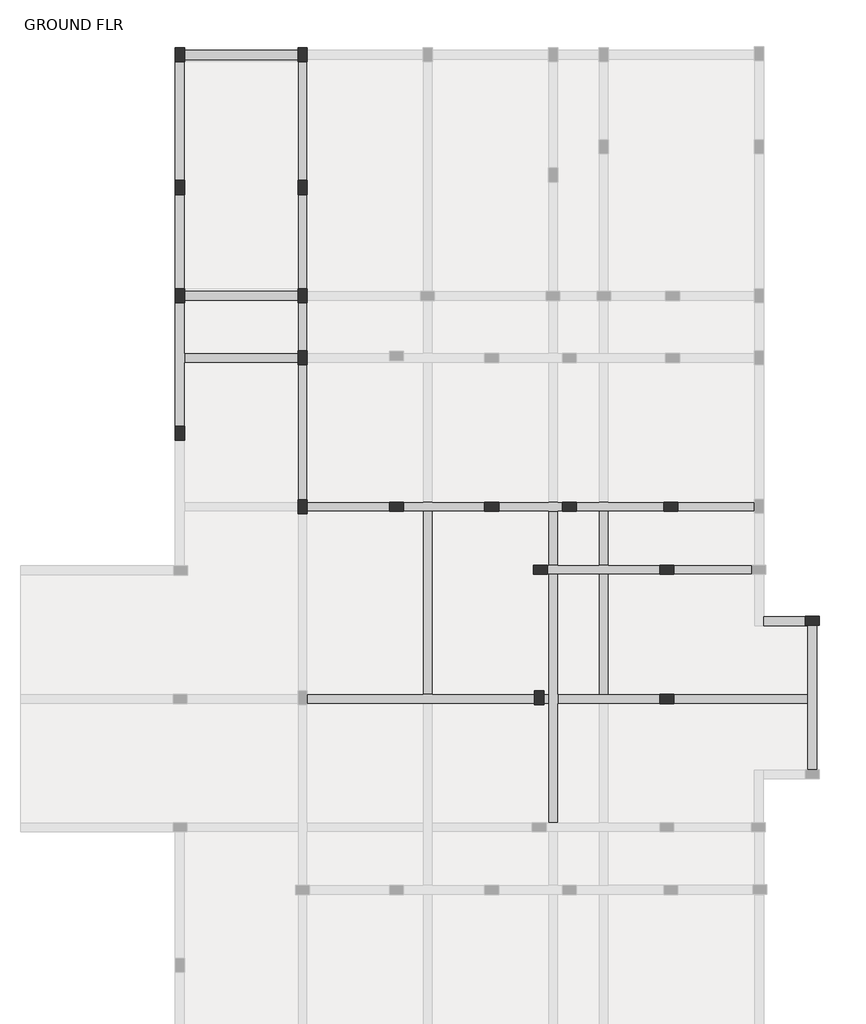
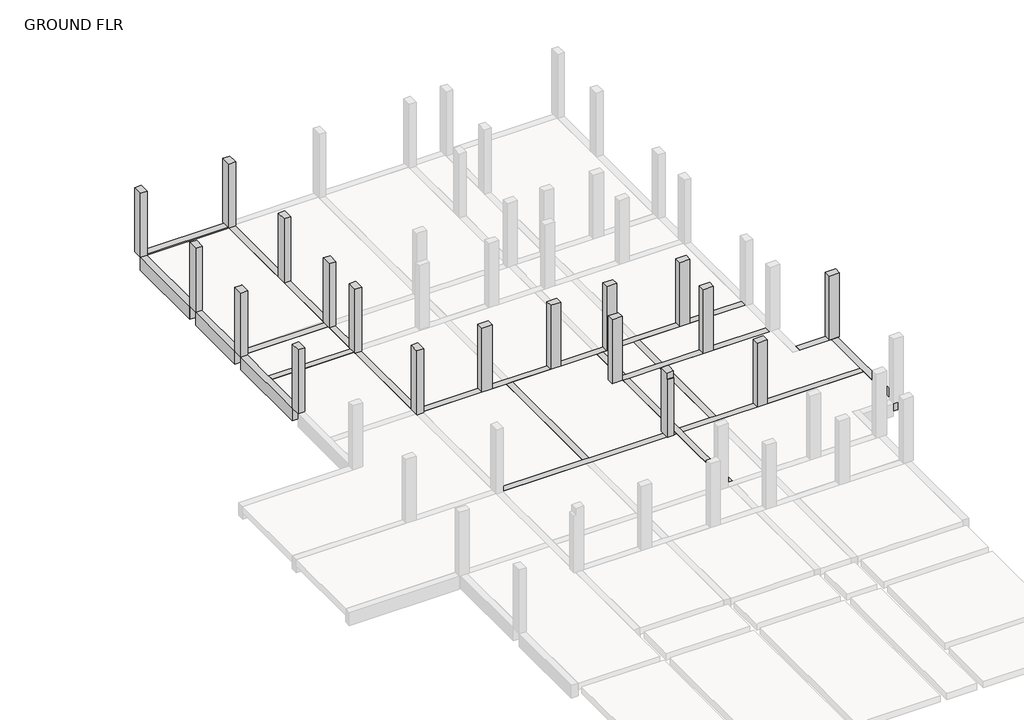
# One storey, part 4 of 5: 29 beams, 18 columns.
"""IFC4 building model written with IfcOpenShell, lengths in millimetres."""

from ifc_helpers import new_model, si_unit, frame, origin, origin_with_axes, place, context, project, spatial, polyline, outline, extrude, faceted_brep, element, save

model = new_model("IFC4")

# Units and contexts
model_context = context("Model", 3, world=origin())
ifc_project = project(units=[si_unit("LENGTHUNIT", "METRE", prefix="MILLI")], contexts=[model_context])

# Site, building, storey
site = spatial("IfcSite", under=ifc_project)
building = spatial("IfcBuilding", under=site)
storey = spatial("IfcBuildingStorey", under=building, Name="GROUND FLR", Elevation=0.0)

# Beams
placement = place(None, origin())
element("IfcBeam", 1, ObjectType="M_Concrete-Rectangular Beam : 300 x 600mm", at=placement, inside=storey, context=model_context, shape_type="SweptSolid", body=[
    extrude(outline(polyline([(-1971.7865686, 21837.8349362), (-1971.7865686, 21537.8349362), (-5591.7865686, 21537.8349362), (-5591.7865686, 21837.8349362), (-1971.7865686, 21837.8349362)])), frame((0.0, 0.0, -600.0), z_axis=(0.0, 0.0, 1.0), x_axis=(1.0, 0.0, 0.0)), (0.0, 0.0, 1.0), 600.0),
])
element("IfcBeam", 2, ObjectType="M_Concrete-Rectangular Beam : 300 x 600mm", at=placement, inside=storey, context=model_context, shape_type="Brep", body=[
    faceted_brep([(-5891.7865686, 21462.8349362, 0.0), (-5891.7865686, 17662.8349362, 0.0), (-5888.8105653, 17662.8349362, 0.0), (-5888.8105653, 17674.7148651, 0.0), (-5591.7865686, 17674.7148651, 0.0), (-5591.7865686, 21462.8349362, 0.0), (-5891.7865686, 21462.8349362, -600.0), (-5891.7865686, 17662.8349362, -600.0), (-5591.7865686, 21462.8349362, -600.0), (-5591.7865686, 17674.7148651, -600.0), (-5888.8105653, 17674.7148651, -600.0), (-5888.8105653, 17662.8349362, -600.0), (-5591.7865686, 17674.7148651, -300.0), (-5591.7865686, 21462.8349362, -300.0)], [[[0, 1, 2, 3, 4, 5]], [[1, 0, 6, 7]], [[7, 6, 8, 9, 10, 11]], [[5, 4, 12, 9, 8, 13]], [[8, 6, 0, 5, 13]], [[1, 7, 11, 2]], [[10, 3, 2, 11]], [[3, 10, 9, 12, 4]]]),
])
element("IfcBeam", 3, ObjectType="M_Concrete-Rectangular Beam : 300 x 600mm", at=placement, inside=storey, context=model_context, shape_type="SweptSolid", body=[
    extrude(outline(polyline([(0.0, -5888.8105653), (-600.0, -5888.8105653), (-600.0, -5588.8105653), (-300.0, -5588.8105653), (-300.0, -5591.7865686), (0.0, -5591.7865686), (0.0, -5888.8105653)])), frame((0.0, 14212.5179708, 0.0), z_axis=(0.0, 1.0, 0.0), x_axis=(0.0, 0.0, 1.0)), (0.0, 0.0, 1.0), 3012.1968944),
])
element("IfcBeam", 4, ObjectType="M_Concrete-Rectangular Beam : 300 x 600mm", at=placement, inside=storey, context=model_context, shape_type="Brep", body=[
    faceted_brep([(-5888.8105653, 13762.5179708, 0.0), (-5888.8105653, 9817.5252033, 0.0), (-5588.8105653, 9817.5252033, 0.0), (-5588.8105653, 11857.4075451, 0.0), (-5588.8105653, 12157.4075451, 0.0), (-5588.8105653, 13762.5179708, 0.0), (-5888.8105653, 13762.5179708, -600.0), (-5888.8105653, 9817.5252033, -600.0), (-5588.8105653, 13762.5179708, -600.0), (-5588.8105653, 12157.4075451, -600.0), (-5588.8105653, 11857.4075451, -600.0), (-5588.8105653, 9817.5252033, -600.0), (-5588.8105653, 13762.5179708, -300.0), (-5588.8105653, 9817.5252033, -300.0)], [[[0, 1, 2, 3, 4, 5]], [[1, 0, 6, 7]], [[7, 6, 8, 9, 10, 11]], [[11, 10, 9, 8, 12, 5, 4, 3, 2, 13]], [[8, 6, 0, 5, 12]], [[2, 1, 7, 11, 13]]]),
])
element("IfcBeam", 5, ObjectType="M_Concrete-Rectangular Beam : 300 x 600mm", at=placement, inside=storey, context=model_context, shape_type="Brep", body=[
    faceted_brep([(14319.1163908, 3443.0536525, 0.0), (14619.1163908, 3443.0536525, 0.0), (14619.1163908, 3443.0536525, -600.0), (14319.1163908, 3443.0536525, -600.0), (14319.1163908, 3435.7536525, 0.0), (14319.1163908, 1251.1713929, 0.0), (14319.1163908, 951.1713929, 0.0), (14319.1163908, -1148.8286071, 0.0), (14619.1163908, -1148.8286071, 0.0), (14619.1163908, -1148.8286071, -600.0), (14319.1163908, -1148.8286071, -600.0), (14319.1163908, 951.1713929, -600.0), (14319.1163908, 1251.1713929, -600.0), (14319.1163908, 3435.7536525, -600.0), (14319.1163908, -1148.8286071, -300.0)], [[[0, 1, 2, 3]], [[1, 0, 4, 5, 6, 7, 8]], [[2, 1, 8, 9]], [[3, 2, 9, 10, 11, 12, 13]], [[0, 3, 13, 12, 11, 10, 14, 7, 6, 5, 4]], [[7, 14, 10, 9, 8]]]),
])
element("IfcBeam", 6, ObjectType="M_Concrete-Rectangular Beam : 300 x 600mm", at=placement, inside=storey, context=model_context, shape_type="Brep", body=[
    faceted_brep([(12916.8679014, 3735.7536525, 0.0), (12916.8679014, 3435.7536525, 0.0), (14319.1163908, 3435.7536525, 0.0), (14319.1163908, 3443.0536525, 0.0), (14619.1163908, 3443.0536525, 0.0), (14619.1163908, 3455.7536525, 0.0), (14244.1163908, 3455.7536525, 0.0), (14244.1163908, 3735.7536525, 0.0), (12916.8679014, 3735.7536525, -600.0), (14244.1163908, 3735.7536525, -600.0), (12916.8679014, 3435.7536525, -600.0), (14244.1163908, 3455.7536525, -600.0), (14619.1163908, 3455.7536525, -600.0), (14619.1163908, 3443.0536525, -600.0), (14319.1163908, 3443.0536525, -600.0), (14319.1163908, 3435.7536525, -600.0), (12916.8679014, 3435.7536525, -300.0), (14319.1163908, 3435.7536525, -300.0)], [[[0, 1, 2, 3, 4, 5, 6, 7]], [[8, 0, 7, 9]], [[10, 8, 9, 11, 12, 13, 14, 15]], [[2, 1, 16, 10, 15, 17]], [[1, 0, 8, 10, 16]], [[12, 5, 4, 13]], [[7, 6, 11, 9]], [[11, 6, 5, 12]], [[3, 14, 13, 4]], [[14, 3, 2, 17, 15]]]),
])
element("IfcBeam", 7, ObjectType="M_Concrete-Rectangular Beam : 300 x 600mm", at=placement, inside=storey, context=model_context, shape_type="Brep", body=[
    faceted_brep([(-1671.7865686, 21462.8349362, 0.0), (-1971.7865686, 21462.8349362, 0.0), (-1971.7865686, 17674.7148651, 0.0), (-1671.7865686, 17674.7148651, 0.0), (-1971.7865686, 21462.8349362, -300.0), (-1971.7865686, 21462.8349362, -600.0), (-1971.7865686, 17674.7148651, -600.0), (-1971.7865686, 17674.7148651, -300.0), (-1671.7865686, 21462.8349362, -600.0), (-1671.7865686, 17674.7148651, -600.0), (-1671.7865686, 17674.7148651, -300.0), (-1671.7865686, 21462.8349362, -300.0)], [[[0, 1, 2, 3]], [[2, 1, 4, 5, 6, 7]], [[5, 8, 9, 6]], [[0, 3, 10, 9, 8, 11]], [[1, 0, 11, 8, 5, 4]], [[3, 2, 7, 6, 9, 10]]]),
])
element("IfcBeam", 8, ObjectType="M_Concrete-Rectangular Beam : 300 x 600mm", at=placement, inside=storey, context=model_context, shape_type="Brep", body=[
    faceted_brep([(-1671.7865686, 17224.7148651, 0.0), (-1971.7865686, 17224.7148651, 0.0), (-1971.7865686, 14212.5179708, 0.0), (-1671.7865686, 14212.5179708, 0.0), (-1971.7865686, 17224.7148651, -300.0), (-1971.7865686, 17224.7148651, -600.0), (-1971.7865686, 14212.5179708, -600.0), (-1971.7865686, 14212.5179708, -300.0), (-1671.7865686, 17224.7148651, -600.0), (-1671.7865686, 14212.5179708, -600.0), (-1671.7865686, 14212.5179708, -300.0), (-1671.7865686, 17224.7148651, -300.0)], [[[0, 1, 2, 3]], [[2, 1, 4, 5, 6, 7]], [[5, 8, 9, 6]], [[0, 3, 10, 9, 8, 11]], [[1, 0, 11, 8, 5, 4]], [[3, 2, 7, 6, 9, 10]]]),
])
element("IfcBeam", 9, ObjectType="M_Concrete-Rectangular Beam : 300 x 600mm", at=placement, inside=storey, context=model_context, shape_type="Brep", body=[
    faceted_brep([(-1671.7865686, 13762.5179708, 0.0), (-1971.7865686, 13762.5179708, 0.0), (-1971.7865686, 12232.4075451, 0.0), (-1671.7865686, 12232.4075451, 0.0), (-1971.7865686, 13762.5179708, -300.0), (-1971.7865686, 13762.5179708, -600.0), (-1971.7865686, 12232.4075451, -600.0), (-1971.7865686, 12232.4075451, -300.0), (-1671.7865686, 13762.5179708, -600.0), (-1671.7865686, 12232.4075451, -600.0), (-1671.7865686, 12232.4075451, -300.0), (-1671.7865686, 13762.5179708, -300.0)], [[[0, 1, 2, 3]], [[2, 1, 4, 5, 6, 7]], [[5, 8, 9, 6]], [[0, 3, 10, 9, 8, 11]], [[1, 0, 11, 8, 5, 4]], [[3, 2, 7, 6, 9, 10]]]),
])
element("IfcBeam", 10, ObjectType="M_Concrete-Rectangular Beam : 300 x 600mm", at=placement, inside=storey, context=model_context, shape_type="Brep", body=[
    faceted_brep([(-1671.7865686, 11782.4075451, 0.0), (-1971.7865686, 11782.4075451, 0.0), (-1971.7865686, 7474.7076276, 0.0), (-1671.7865686, 7474.7076276, 0.0), (-1971.7865686, 11782.4075451, -300.0), (-1971.7865686, 11782.4075451, -600.0), (-1971.7865686, 7474.7076276, -600.0), (-1971.7865686, 7474.7076276, -300.0), (-1671.7865686, 11782.4075451, -600.0), (-1671.7865686, 7474.7076276, -600.0), (-1671.7865686, 7474.7076276, -300.0), (-1671.7865686, 11782.4075451, -300.0)], [[[0, 1, 2, 3]], [[2, 1, 4, 5, 6, 7]], [[5, 8, 9, 6]], [[0, 3, 10, 9, 8, 11]], [[1, 0, 11, 8, 5, 4]], [[3, 2, 7, 6, 9, 10]]]),
])
element("IfcBeam", 11, ObjectType="M_Concrete-Rectangular Beam : 300 x 600mm", at=placement, inside=storey, context=model_context, shape_type="Brep", body=[
    faceted_brep([(-5588.8105653, 14137.5179708, 0.0), (-5588.8105653, 13837.5179708, 0.0), (-1971.7865686, 13837.5179708, 0.0), (-1971.7865686, 14137.5179708, 0.0), (-5588.8105653, 13837.5179708, -300.0), (-5588.8105653, 13837.5179708, -600.0), (-1971.7865686, 13837.5179708, -600.0), (-1971.7865686, 13837.5179708, -300.0), (-5588.8105653, 14137.5179708, -600.0), (-1971.7865686, 14137.5179708, -600.0)], [[[0, 1, 2, 3]], [[2, 1, 4, 5, 6, 7]], [[5, 8, 9, 6]], [[8, 0, 3, 9]], [[1, 0, 8, 5, 4]], [[9, 3, 2, 7, 6]]]),
])
element("IfcBeam", 12, ObjectType="M_Concrete-Rectangular Beam : 300 x 600mm", at=placement, inside=storey, context=model_context, shape_type="Brep", body=[
    faceted_brep([(-1971.7865686, 11857.4075451, 0.0), (-1971.7865686, 12157.4075451, 0.0), (-5588.8105653, 12157.4075451, 0.0), (-5588.8105653, 11857.4075451, 0.0), (-5588.8105653, 11857.4075451, -300.0), (-5588.8105653, 11857.4075451, -600.0), (-1971.7865686, 11857.4075451, -600.0), (-1971.7865686, 11857.4075451, -300.0), (-1971.7865686, 12157.4075451, -600.0), (-5588.8105653, 12157.4075451, -600.0), (-1971.7865686, 12157.4075451, -300.0), (-5588.8105653, 12157.4075451, -300.0)], [[[0, 1, 2, 3]], [[0, 3, 4, 5, 6, 7]], [[8, 6, 5, 9]], [[2, 1, 10, 8, 9, 11]], [[1, 0, 7, 6, 8, 10]], [[3, 2, 11, 9, 5, 4]]]),
])
element("IfcBeam", 13, ObjectType="M_Concrete-Rectangular Beam : 300 x 600mm", at=placement, inside=storey, context=model_context, shape_type="Brep", body=[
    faceted_brep([(-1671.7865686, 7399.7076276, 0.0), (-1671.7865686, 7099.7076276, 0.0), (949.7296816, 7099.7076276, 0.0), (949.7296816, 7399.7076276, 0.0), (-1671.7865686, 7099.7076276, -300.0), (-1671.7865686, 7099.7076276, -600.0), (949.7296816, 7099.7076276, -600.0), (949.7296816, 7099.7076276, -300.0), (-1671.7865686, 7399.7076276, -600.0), (949.7296816, 7399.7076276, -600.0), (949.7296816, 7399.7076276, -300.0), (-1671.7865686, 7399.7076276, -300.0)], [[[0, 1, 2, 3]], [[2, 1, 4, 5, 6, 7]], [[5, 8, 9, 6]], [[0, 3, 10, 9, 8, 11]], [[1, 0, 11, 8, 5, 4]], [[3, 2, 7, 6, 9, 10]]]),
])
element("IfcBeam", 14, ObjectType="M_Concrete-Rectangular Beam : 300 x 600mm", at=placement, inside=storey, context=model_context, shape_type="Brep", body=[
    faceted_brep([(1399.7296816, 7399.7076276, 0.0), (1399.7296816, 7099.7076276, 0.0), (2024.7296816, 7099.7076276, 0.0), (2324.7296816, 7099.7076276, 0.0), (3997.5248054, 7099.7076276, 0.0), (3997.5248054, 7399.7076276, 0.0), (2324.7296816, 7399.7076276, 0.0), (2024.7296816, 7399.7076276, 0.0), (1399.7296816, 7099.7076276, -600.0), (2024.7296816, 7099.7076276, -600.0), (2324.7296816, 7099.7076276, -600.0), (3997.5248054, 7099.7076276, -600.0), (3997.5248054, 7099.7076276, -300.0), (1399.7296816, 7099.7076276, -300.0), (1399.7296816, 7399.7076276, -600.0), (2024.7296816, 7399.7076276, -600.0), (2324.7296816, 7399.7076276, -600.0), (3997.5248054, 7399.7076276, -600.0), (1399.7296816, 7399.7076276, -300.0), (3997.5248054, 7399.7076276, -300.0)], [[[0, 1, 2, 3, 4, 5, 6, 7]], [[8, 9, 10, 11, 12, 4, 3, 2, 1, 13]], [[8, 14, 15, 16, 17, 11, 10, 9]], [[17, 16, 15, 14, 18, 0, 7, 6, 5, 19]], [[1, 0, 18, 14, 8, 13]], [[5, 4, 12, 11, 17, 19]]]),
])
element("IfcBeam", 15, ObjectType="M_Concrete-Rectangular Beam : 300 x 600mm", at=placement, inside=storey, context=model_context, shape_type="Brep", body=[
    faceted_brep([(4447.5248054, 7399.7076276, 0.0), (4447.5248054, 7099.7076276, 0.0), (6032.5248054, 7099.7076276, 0.0), (6332.5248054, 7099.7076276, 0.0), (6481.8679014, 7099.7076276, 0.0), (6481.8679014, 7399.7076276, 0.0), (6332.5248054, 7399.7076276, 0.0), (6032.5248054, 7399.7076276, 0.0), (4447.5248054, 7099.7076276, -600.0), (6032.5248054, 7099.7076276, -600.0), (6332.5248054, 7099.7076276, -600.0), (6481.8679014, 7099.7076276, -600.0), (6481.8679014, 7099.7076276, -300.0), (4447.5248054, 7099.7076276, -300.0), (4447.5248054, 7399.7076276, -600.0), (6032.5248054, 7399.7076276, -600.0), (6332.5248054, 7399.7076276, -600.0), (6481.8679014, 7399.7076276, -600.0), (4447.5248054, 7399.7076276, -300.0), (6481.8679014, 7399.7076276, -300.0)], [[[0, 1, 2, 3, 4, 5, 6, 7]], [[8, 9, 10, 11, 12, 4, 3, 2, 1, 13]], [[8, 14, 15, 16, 17, 11, 10, 9]], [[17, 16, 15, 14, 18, 0, 7, 6, 5, 19]], [[1, 0, 18, 14, 8, 13]], [[5, 4, 12, 11, 17, 19]]]),
])
element("IfcBeam", 16, ObjectType="M_Concrete-Rectangular Beam : 300 x 600mm", at=placement, inside=storey, context=model_context, shape_type="Brep", body=[
    faceted_brep([(6931.8679014, 7399.7076276, 0.0), (6931.8679014, 7099.7076276, 0.0), (7656.8679014, 7099.7076276, 0.0), (7956.8679014, 7099.7076276, 0.0), (9721.8679014, 7099.7076276, 0.0), (9721.8679014, 7399.7076276, 0.0), (7956.8679014, 7399.7076276, 0.0), (7656.8679014, 7399.7076276, 0.0), (6931.8679014, 7099.7076276, -600.0), (7656.8679014, 7099.7076276, -600.0), (7956.8679014, 7099.7076276, -600.0), (9721.8679014, 7099.7076276, -600.0), (9721.8679014, 7099.7076276, -300.0), (6931.8679014, 7099.7076276, -300.0), (6931.8679014, 7399.7076276, -600.0), (7656.8679014, 7399.7076276, -600.0), (7956.8679014, 7399.7076276, -600.0), (9721.8679014, 7399.7076276, -600.0), (6931.8679014, 7399.7076276, -300.0), (9721.8679014, 7399.7076276, -300.0)], [[[0, 1, 2, 3, 4, 5, 6, 7]], [[8, 9, 10, 11, 12, 4, 3, 2, 1, 13]], [[8, 14, 15, 16, 17, 11, 10, 9]], [[17, 16, 15, 14, 18, 0, 7, 6, 5, 19]], [[1, 0, 18, 14, 8, 13]], [[5, 4, 12, 11, 17, 19]]]),
])
element("IfcBeam", 17, ObjectType="M_Concrete-Rectangular Beam : 300 x 600mm", at=placement, inside=storey, context=model_context, shape_type="Brep", body=[
    faceted_brep([(6007.5248054, 5387.6057249, 0.0), (6007.5248054, 5087.6057249, 0.0), (6032.5248054, 5087.6057249, 0.0), (6332.5248054, 5087.6057249, 0.0), (7656.8679014, 5087.6057249, 0.0), (7956.8679014, 5087.6057249, 0.0), (9601.8679014, 5087.6057249, 0.0), (9601.8679014, 5387.6057249, 0.0), (7956.8679014, 5387.6057249, 0.0), (7656.8679014, 5387.6057249, 0.0), (6332.5248054, 5387.6057249, 0.0), (6032.5248054, 5387.6057249, 0.0), (6007.5248054, 5087.6057249, -600.0), (6032.5248054, 5087.6057249, -600.0), (6332.5248054, 5087.6057249, -600.0), (7656.8679014, 5087.6057249, -600.0), (7956.8679014, 5087.6057249, -600.0), (9601.8679014, 5087.6057249, -600.0), (9601.8679014, 5087.6057249, -300.0), (6007.5248054, 5087.6057249, -300.0), (6007.5248054, 5387.6057249, -600.0), (6032.5248054, 5387.6057249, -600.0), (6332.5248054, 5387.6057249, -600.0), (7656.8679014, 5387.6057249, -600.0), (7956.8679014, 5387.6057249, -600.0), (9601.8679014, 5387.6057249, -600.0), (6007.5248054, 5387.6057249, -300.0), (9601.8679014, 5387.6057249, -300.0)], [[[0, 1, 2, 3, 4, 5, 6, 7, 8, 9, 10, 11]], [[12, 13, 14, 15, 16, 17, 18, 6, 5, 4, 3, 2, 1, 19]], [[12, 20, 21, 22, 23, 24, 25, 17, 16, 15, 14, 13]], [[25, 24, 23, 22, 21, 20, 26, 0, 11, 10, 9, 8, 7, 27]], [[1, 0, 26, 20, 12, 19]], [[7, 6, 18, 17, 25, 27]]]),
])
element("IfcBeam", 18, ObjectType="M_Concrete-Rectangular Beam : 300 x 600mm", at=placement, inside=storey, context=model_context, shape_type="Brep", body=[
    faceted_brep([(10051.8679014, 5387.6057249, 0.0), (10051.8679014, 5087.6057249, 0.0), (12541.8679014, 5087.6057249, 0.0), (12541.8679014, 5387.6057249, 0.0), (10051.8679014, 5087.6057249, -300.0), (10051.8679014, 5087.6057249, -600.0), (12541.8679014, 5087.6057249, -600.0), (12541.8679014, 5087.6057249, -300.0), (10051.8679014, 5387.6057249, -600.0), (12541.8679014, 5387.6057249, -600.0), (12541.8679014, 5387.6057249, -300.0), (10051.8679014, 5387.6057249, -300.0)], [[[0, 1, 2, 3]], [[2, 1, 4, 5, 6, 7]], [[5, 8, 9, 6]], [[0, 3, 10, 9, 8, 11]], [[1, 0, 11, 8, 5, 4]], [[3, 2, 7, 6, 9, 10]]]),
])
element("IfcBeam", 19, ObjectType="M_Concrete-Rectangular Beam : 300 x 600mm", at=placement, inside=storey, context=model_context, shape_type="Brep", body=[
    faceted_brep([(10051.8679014, 1251.1713929, 0.0), (10051.8679014, 951.1713929, 0.0), (14319.1163908, 951.1713929, 0.0), (14319.1163908, 1251.1713929, 0.0), (10051.8679014, 951.1713929, -300.0), (10051.8679014, 951.1713929, -600.0), (14319.1163908, 951.1713929, -600.0), (14319.1163908, 951.1713929, -300.0), (10051.8679014, 1251.1713929, -600.0), (14319.1163908, 1251.1713929, -600.0), (14319.1163908, 1251.1713929, -300.0), (10051.8679014, 1251.1713929, -300.0)], [[[0, 1, 2, 3]], [[2, 1, 4, 5, 6, 7]], [[5, 8, 9, 6]], [[0, 3, 10, 9, 8, 11]], [[1, 0, 11, 8, 5, 4]], [[3, 2, 7, 6, 9, 10]]]),
])
element("IfcBeam", 20, ObjectType="M_Concrete-Rectangular Beam : 300 x 600mm", at=placement, inside=storey, context=model_context, shape_type="Brep", body=[
    faceted_brep([(6032.5248054, 951.1713929, 0.0), (6032.5248054, 1251.1713929, 0.0), (5892.5248054, 1251.1713929, 0.0), (5892.5248054, 951.1713929, 0.0), (5892.5248054, 951.1713929, -300.0), (5892.5248054, 951.1713929, -600.0), (6032.5248054, 951.1713929, -600.0), (6032.5248054, 951.1713929, -300.0), (6032.5248054, 1251.1713929, -600.0), (5892.5248054, 1251.1713929, -600.0), (6032.5248054, 1251.1713929, -300.0), (5892.5248054, 1251.1713929, -300.0)], [[[0, 1, 2, 3]], [[0, 3, 4, 5, 6, 7]], [[8, 6, 5, 9]], [[2, 1, 10, 8, 9, 11]], [[1, 0, 7, 6, 8, 10]], [[3, 2, 11, 9, 5, 4]]]),
    faceted_brep([(-1671.7865686, 951.1713929, 0.0), (-1671.7865686, 1251.1713929, 0.0), (-1671.7865686, 1251.1713929, -300.0), (-1671.7865686, 1251.1713929, -600.0), (-1671.7865686, 951.1713929, -600.0), (-1671.7865686, 951.1713929, -300.0), (5592.5248054, 1251.1713929, 0.0), (5592.5248054, 951.1713929, 0.0), (5592.5248054, 951.1713929, -300.0), (5592.5248054, 951.1713929, -600.0), (5592.5248054, 1251.1713929, -600.0), (5592.5248054, 1251.1713929, -300.0), (2024.7296816, 951.1713929, 0.0), (2324.7296816, 951.1713929, 0.0), (2324.7296816, 1251.1713929, 0.0), (2024.7296816, 1251.1713929, 0.0), (2024.7296816, 951.1713929, -600.0), (2324.7296816, 951.1713929, -600.0), (2024.7296816, 1251.1713929, -600.0), (2324.7296816, 1251.1713929, -600.0)], [[[0, 1, 2, 3, 4, 5]], [[6, 7, 8, 9, 10, 11]], [[1, 0, 12, 13, 7, 6, 14, 15]], [[4, 16, 17, 9, 8, 7, 13, 12, 0, 5]], [[4, 3, 18, 19, 10, 9, 17, 16]], [[10, 19, 18, 3, 2, 1, 15, 14, 6, 11]]]),
])
element("IfcBeam", 21, ObjectType="M_Concrete-Rectangular Beam : 300 x 600mm", at=placement, inside=storey, context=model_context, shape_type="Brep", body=[
    faceted_brep([(2324.7296816, 7099.7076276, 0.0), (2024.7296816, 7099.7076276, 0.0), (2024.7296816, 1251.1713929, 0.0), (2324.7296816, 1251.1713929, 0.0), (2024.7296816, 7099.7076276, -300.0), (2024.7296816, 7099.7076276, -600.0), (2024.7296816, 1251.1713929, -600.0), (2024.7296816, 1251.1713929, -300.0), (2324.7296816, 7099.7076276, -600.0), (2324.7296816, 5387.6057249, -600.0), (2324.7296816, 5087.6057249, -600.0), (2324.7296816, 1251.1713929, -600.0), (2324.7296816, 1251.1713929, -300.0), (2324.7296816, 7099.7076276, -300.0)], [[[0, 1, 2, 3]], [[2, 1, 4, 5, 6, 7]], [[5, 8, 9, 10, 11, 6]], [[0, 3, 12, 11, 10, 9, 8, 13]], [[1, 0, 13, 8, 5, 4]], [[3, 2, 7, 6, 11, 12]]]),
])
element("IfcBeam", 22, ObjectType="M_Concrete-Rectangular Beam : 300 x 600mm", at=placement, inside=storey, context=model_context, shape_type="Brep", body=[
    faceted_brep([(6332.5248054, 7099.7076276, 0.0), (6032.5248054, 7099.7076276, 0.0), (6032.5248054, 5387.6057249, 0.0), (6332.5248054, 5387.6057249, 0.0), (6032.5248054, 7099.7076276, -300.0), (6032.5248054, 7099.7076276, -600.0), (6032.5248054, 5387.6057249, -600.0), (6032.5248054, 5387.6057249, -300.0), (6332.5248054, 7099.7076276, -600.0), (6332.5248054, 5387.6057249, -600.0), (6332.5248054, 5387.6057249, -300.0), (6332.5248054, 7099.7076276, -300.0)], [[[0, 1, 2, 3]], [[2, 1, 4, 5, 6, 7]], [[5, 8, 9, 6]], [[0, 3, 10, 9, 8, 11]], [[1, 0, 11, 8, 5, 4]], [[3, 2, 7, 6, 9, 10]]]),
])
element("IfcBeam", 23, ObjectType="M_Concrete-Rectangular Beam : 300 x 600mm", at=placement, inside=storey, context=model_context, shape_type="Brep", body=[
    faceted_brep([(7956.8679014, 7099.7076276, 0.0), (7656.8679014, 7099.7076276, 0.0), (7656.8679014, 5387.6057249, 0.0), (7956.8679014, 5387.6057249, 0.0), (7656.8679014, 7099.7076276, -300.0), (7656.8679014, 7099.7076276, -600.0), (7656.8679014, 5387.6057249, -600.0), (7656.8679014, 5387.6057249, -300.0), (7956.8679014, 7099.7076276, -600.0), (7956.8679014, 5387.6057249, -600.0), (7956.8679014, 5387.6057249, -300.0), (7956.8679014, 7099.7076276, -300.0)], [[[0, 1, 2, 3]], [[2, 1, 4, 5, 6, 7]], [[5, 8, 9, 6]], [[0, 3, 10, 9, 8, 11]], [[1, 0, 11, 8, 5, 4]], [[3, 2, 7, 6, 9, 10]]]),
])
element("IfcBeam", 24, ObjectType="M_Concrete-Rectangular Beam : 300 x 600mm", at=placement, inside=storey, context=model_context, shape_type="Brep", body=[
    faceted_brep([(6332.5248054, 5087.6057249, 0.0), (6032.5248054, 5087.6057249, 0.0), (6032.5248054, 1251.1713929, 0.0), (6032.5248054, 951.1713929, 0.0), (6032.5248054, -2839.4535766, 0.0), (6332.5248054, -2839.4535766, 0.0), (6332.5248054, 951.1713929, 0.0), (6332.5248054, 1251.1713929, 0.0), (6032.5248054, 5087.6057249, -600.0), (6032.5248054, 1251.1713929, -600.0), (6032.5248054, 951.1713929, -600.0), (6032.5248054, -2839.4535766, -600.0), (6032.5248054, -2839.4535766, -300.0), (6032.5248054, 5087.6057249, -300.0), (6332.5248054, 5087.6057249, -600.0), (6332.5248054, 1251.1713929, -600.0), (6332.5248054, 951.1713929, -600.0), (6332.5248054, -2839.4535766, -600.0), (6332.5248054, 5087.6057249, -300.0), (6332.5248054, -2839.4535766, -300.0)], [[[0, 1, 2, 3, 4, 5, 6, 7]], [[8, 9, 10, 11, 12, 4, 3, 2, 1, 13]], [[8, 14, 15, 16, 17, 11, 10, 9]], [[17, 16, 15, 14, 18, 0, 7, 6, 5, 19]], [[1, 0, 18, 14, 8, 13]], [[5, 4, 12, 11, 17, 19]]]),
])
element("IfcBeam", 25, ObjectType="M_Concrete-Rectangular Beam : 300 x 600mm", at=placement, inside=storey, context=model_context, shape_type="Brep", body=[
    faceted_brep([(7956.8679014, 5087.6057249, 0.0), (7656.8679014, 5087.6057249, 0.0), (7656.8679014, 1251.1713929, 0.0), (7956.8679014, 1251.1713929, 0.0), (7656.8679014, 5087.6057249, -300.0), (7656.8679014, 5087.6057249, -600.0), (7656.8679014, 1251.1713929, -600.0), (7656.8679014, 1251.1713929, -300.0), (7956.8679014, 5087.6057249, -600.0), (7956.8679014, 1251.1713929, -600.0), (7956.8679014, 1251.1713929, -300.0), (7956.8679014, 5087.6057249, -300.0)], [[[0, 1, 2, 3]], [[2, 1, 4, 5, 6, 7]], [[5, 8, 9, 6]], [[0, 3, 10, 9, 8, 11]], [[1, 0, 11, 8, 5, 4]], [[3, 2, 7, 6, 9, 10]]]),
])
element("IfcBeam", 26, ObjectType="M_Concrete-Rectangular Beam : 300 x 600mm", at=placement, inside=storey, context=model_context, shape_type="Brep", body=[
    faceted_brep([(9601.8679014, 951.1713929, 0.0), (9601.8679014, 1251.1713929, 0.0), (7956.8679014, 1251.1713929, 0.0), (7656.8679014, 1251.1713929, 0.0), (6332.5248054, 1251.1713929, 0.0), (6332.5248054, 951.1713929, 0.0), (7656.8679014, 951.1713929, 0.0), (7956.8679014, 951.1713929, 0.0), (6332.5248054, 951.1713929, -600.0), (7656.8679014, 951.1713929, -600.0), (7956.8679014, 951.1713929, -600.0), (9601.8679014, 951.1713929, -600.0), (9601.8679014, 951.1713929, -300.0), (6332.5248054, 951.1713929, -300.0), (9601.8679014, 1251.1713929, -600.0), (6332.5248054, 1251.1713929, -600.0), (7656.8679014, 1251.1713929, -600.0), (7956.8679014, 1251.1713929, -600.0), (6332.5248054, 1251.1713929, -300.0), (9601.8679014, 1251.1713929, -300.0)], [[[0, 1, 2, 3, 4, 5, 6, 7]], [[8, 9, 10, 11, 12, 0, 7, 6, 5, 13]], [[14, 11, 10, 9, 8, 15, 16, 17]], [[14, 17, 16, 15, 18, 4, 3, 2, 1, 19]], [[1, 0, 12, 11, 14, 19]], [[5, 4, 18, 15, 8, 13]]]),
])
element("IfcBeam", 27, ObjectType="M_Concrete-Rectangular Beam : 300 x 600mm", at=placement, inside=storey, context=model_context, shape_type="Brep", body=[
    faceted_brep([(10171.8679014, 7399.7076276, 0.0), (10171.8679014, 7099.7076276, 0.0), (12616.8679014, 7099.7076276, 0.0), (12616.8679014, 7399.7076276, 0.0), (10171.8679014, 7099.7076276, -300.0), (10171.8679014, 7099.7076276, -600.0), (12616.8679014, 7099.7076276, -600.0), (12616.8679014, 7099.7076276, -300.0), (10171.8679014, 7399.7076276, -600.0), (12616.8679014, 7399.7076276, -600.0), (12616.8679014, 7399.7076276, -300.0), (10171.8679014, 7399.7076276, -300.0)], [[[0, 1, 2, 3]], [[2, 1, 4, 5, 6, 7]], [[5, 8, 9, 6]], [[0, 3, 10, 9, 8, 11]], [[8, 5, 4, 1, 0, 11]], [[3, 2, 7, 6, 9, 10]]]),
])
element("IfcBeam", 28, ObjectType="M_Concrete-Rectangular Beam : 300 x 600mm", at=placement, inside=storey, context=model_context, shape_type="SweptSolid", body=[
    extrude(outline(polyline([(2324.7296816, 5087.6057249), (2324.7296816, 5387.6057249), (2337.5248054, 5387.6057249), (2337.5248054, 5087.6057249), (2324.7296816, 5087.6057249)])), frame((0.0, 0.0, -600.0), z_axis=(0.0, 0.0, 1.0), x_axis=(1.0, 0.0, 0.0)), (0.0, 0.0, 1.0), 300.0),
])
element("IfcBeam", 29, ObjectType="M_Concrete-Rectangular Beam : 300 x 600mm", at=placement, inside=storey, context=model_context, shape_type="SweptSolid", body=[
    extrude(outline(polyline([(2337.5248054, 5087.6057249), (2337.5248054, 5387.6057249), (5557.5248054, 5387.6057249), (5557.5248054, 5087.6057249), (2337.5248054, 5087.6057249)])), frame((0.0, 0.0, -600.0), z_axis=(0.0, 0.0, 1.0), x_axis=(1.0, 0.0, 0.0)), (0.0, 0.0, 1.0), 300.0),
])

# Columns
element("IfcColumn", 30, ObjectType="M_Concrete-Rectangular-Column : 300 x 450mm", at=placement, inside=storey, context=model_context, shape_type="SweptSolid", body=[
    extrude(outline(polyline([(-5591.7865686, 21912.8349362), (-5591.7865686, 21462.8349362), (-5891.7865686, 21462.8349362), (-5891.7865686, 21912.8349362), (-5591.7865686, 21912.8349362)])), origin_with_axes(), (0.0, 0.0, 1.0), 3000.0),
])
element("IfcColumn", 31, ObjectType="M_Concrete-Rectangular-Column : 300 x 450mm", at=placement, inside=storey, context=model_context, shape_type="Brep", body=[
    faceted_brep([(-1671.7865686, 21912.8349362, 0.0), (-1671.7865686, 21462.8349362, 0.0), (-1971.7865686, 21462.8349362, 0.0), (-1971.7865686, 21912.8349362, 0.0), (-1671.7865686, 21912.8349362, 3000.0), (-1671.7865686, 21537.8349362, 3000.0), (-1671.7865686, 21462.8349362, 3000.0), (-1671.7865686, 21462.8349362, 2700.0), (-1971.7865686, 21462.8349362, 3000.0), (-1971.7865686, 21462.8349362, 2700.0), (-1971.7865686, 21912.8349362, 3000.0)], [[[0, 1, 2, 3]], [[1, 0, 4, 5, 6, 7]], [[2, 1, 7, 6, 8, 9]], [[3, 2, 9, 8, 10]], [[0, 3, 10, 4]], [[8, 6, 5, 4, 10]]]),
])
element("IfcColumn", 32, ObjectType="M_Concrete-Rectangular-Column : 300 x 450mm", at=placement, inside=storey, context=model_context, shape_type="Brep", body=[
    faceted_brep([(-1671.7865686, 17674.7148651, 0.0), (-1671.7865686, 17224.7148651, 0.0), (-1971.7865686, 17224.7148651, 0.0), (-1971.7865686, 17674.7148651, 0.0), (-1671.7865686, 17674.7148651, 2700.0), (-1671.7865686, 17674.7148651, 3000.0), (-1671.7865686, 17224.7148651, 3000.0), (-1671.7865686, 17224.7148651, 2700.0), (-1971.7865686, 17224.7148651, 3000.0), (-1971.7865686, 17224.7148651, 2700.0), (-1971.7865686, 17674.7148651, 3000.0), (-1971.7865686, 17674.7148651, 2700.0)], [[[0, 1, 2, 3]], [[1, 0, 4, 5, 6, 7]], [[2, 1, 7, 6, 8, 9]], [[3, 2, 9, 8, 10, 11]], [[0, 3, 11, 10, 5, 4]], [[6, 5, 10, 8]]]),
])
element("IfcColumn", 33, ObjectType="M_Concrete-Rectangular-Column : 300 x 450mm", at=placement, inside=storey, context=model_context, shape_type="SweptSolid", body=[
    extrude(outline(polyline([(0.0, -5888.8105653), (0.0, -5588.8105653), (2700.0, -5588.8105653), (2700.0, -5591.7865686), (3000.0, -5591.7865686), (3000.0, -5888.8105653), (0.0, -5888.8105653)])), frame((0.0, 17224.7148651, 0.0), z_axis=(0.0, 1.0, 0.0), x_axis=(0.0, 0.0, 1.0)), (0.0, 0.0, 1.0), 450.0),
])
element("IfcColumn", 34, ObjectType="M_Concrete-Rectangular-Column : 300 x 450mm", at=placement, inside=storey, context=model_context, shape_type="Brep", body=[
    faceted_brep([(-5588.8105653, 14212.5179708, 0.0), (-5588.8105653, 13762.5179708, 0.0), (-5888.8105653, 13762.5179708, 0.0), (-5888.8105653, 14212.5179708, 0.0), (-5588.8105653, 14212.5179708, 2700.0), (-5588.8105653, 14212.5179708, 3000.0), (-5588.8105653, 13837.5179708, 3000.0), (-5588.8105653, 13762.5179708, 3000.0), (-5588.8105653, 13762.5179708, 2700.0), (-5888.8105653, 13762.5179708, 3000.0), (-5888.8105653, 14212.5179708, 3000.0), (-5591.7865686, 14212.5179708, 3000.0)], [[[0, 1, 2, 3]], [[1, 0, 4, 5, 6, 7, 8]], [[2, 1, 8, 7, 9]], [[3, 2, 9, 10]], [[0, 3, 10, 11, 5, 4]], [[9, 7, 6, 5, 11, 10]]]),
])
element("IfcColumn", 35, ObjectType="M_Concrete-Rectangular-Column : 300 x 450mm", at=placement, inside=storey, context=model_context, shape_type="Brep", body=[
    faceted_brep([(-1671.7865686, 14212.5179708, 0.0), (-1671.7865686, 13762.5179708, 0.0), (-1971.7865686, 13762.5179708, 0.0), (-1971.7865686, 14212.5179708, 0.0), (-1671.7865686, 14212.5179708, 2700.0), (-1671.7865686, 14212.5179708, 3000.0), (-1671.7865686, 14137.5179708, 3000.0), (-1671.7865686, 13837.5179708, 3000.0), (-1671.7865686, 13762.5179708, 3000.0), (-1671.7865686, 13762.5179708, 2700.0), (-1971.7865686, 13762.5179708, 3000.0), (-1971.7865686, 13762.5179708, 2700.0), (-1971.7865686, 13837.5179708, 3000.0), (-1971.7865686, 14212.5179708, 3000.0), (-1971.7865686, 14212.5179708, 2700.0)], [[[0, 1, 2, 3]], [[1, 0, 4, 5, 6, 7, 8, 9]], [[2, 1, 9, 8, 10, 11]], [[3, 2, 11, 10, 12, 13, 14]], [[0, 3, 14, 13, 5, 4]], [[10, 8, 7, 6, 5, 13, 12]]]),
])
element("IfcColumn", 36, ObjectType="M_Concrete-Rectangular-Column : 300 x 450mm", at=placement, inside=storey, context=model_context, shape_type="Brep", body=[
    faceted_brep([(-1971.7865686, 11782.4075451, 0.0), (-1971.7865686, 12232.4075451, 0.0), (-1671.7865686, 12232.4075451, 0.0), (-1671.7865686, 11782.4075451, 0.0), (-1971.7865686, 11782.4075451, 2700.0), (-1971.7865686, 11782.4075451, 3000.0), (-1971.7865686, 11857.4075451, 3000.0), (-1971.7865686, 12157.4075451, 3000.0), (-1971.7865686, 12232.4075451, 3000.0), (-1971.7865686, 12232.4075451, 2700.0), (-1671.7865686, 12232.4075451, 3000.0), (-1671.7865686, 12232.4075451, 2700.0), (-1671.7865686, 12157.4075451, 3000.0), (-1671.7865686, 11857.4075451, 3000.0), (-1671.7865686, 11782.4075451, 3000.0), (-1671.7865686, 11782.4075451, 2700.0)], [[[0, 1, 2, 3]], [[1, 0, 4, 5, 6, 7, 8, 9]], [[2, 1, 9, 8, 10, 11]], [[3, 2, 11, 10, 12, 13, 14, 15]], [[0, 3, 15, 14, 5, 4]], [[10, 8, 7, 6, 5, 14, 13, 12]]]),
])
element("IfcColumn", 37, ObjectType="M_Concrete-Rectangular-Column : 300 x 450mm", at=placement, inside=storey, context=model_context, shape_type="Brep", body=[
    faceted_brep([(-5888.8105653, 9367.5252033, 0.0), (-5888.8105653, 9817.5252033, 0.0), (-5588.8105653, 9817.5252033, 0.0), (-5588.8105653, 9367.5252033, 0.0), (-5888.8105653, 9367.5252033, 3000.0), (-5888.8105653, 9817.5252033, 3000.0), (-5588.8105653, 9817.5252033, 3000.0), (-5588.8105653, 9817.5252033, 2700.0), (-5588.8105653, 9367.5252033, 3000.0), (-5588.8105653, 9367.5252033, 2700.0)], [[[0, 1, 2, 3]], [[1, 0, 4, 5]], [[2, 1, 5, 6, 7]], [[3, 2, 7, 6, 8, 9]], [[0, 3, 9, 8, 4]], [[5, 4, 8, 6]]]),
])
element("IfcColumn", 38, ObjectType="M_Concrete-Rectangular-Column : 300 x 450mm", at=placement, inside=storey, context=model_context, shape_type="Brep", body=[
    faceted_brep([(-1971.7865686, 7024.7076276, 0.0), (-1971.7865686, 7474.7076276, 0.0), (-1671.7865686, 7474.7076276, 0.0), (-1671.7865686, 7024.7076276, 0.0), (-1971.7865686, 7024.7076276, 2700.0), (-1971.7865686, 7024.7076276, 3000.0), (-1971.7865686, 7099.7076276, 3000.0), (-1971.7865686, 7399.7076276, 3000.0), (-1971.7865686, 7474.7076276, 3000.0), (-1971.7865686, 7474.7076276, 2700.0), (-1671.7865686, 7474.7076276, 3000.0), (-1671.7865686, 7474.7076276, 2700.0), (-1671.7865686, 7399.7076276, 3000.0), (-1671.7865686, 7099.7076276, 3000.0), (-1671.7865686, 7024.7076276, 3000.0), (-1671.7865686, 7024.7076276, 2700.0)], [[[0, 1, 2, 3]], [[1, 0, 4, 5, 6, 7, 8, 9]], [[2, 1, 9, 8, 10, 11]], [[3, 2, 11, 10, 12, 13, 14, 15]], [[0, 3, 15, 14, 5, 4]], [[10, 8, 7, 6, 5, 14, 13, 12]]]),
])
element("IfcColumn", 39, ObjectType="M_Concrete-Rectangular-Column : 300 x 450mm", at=placement, inside=storey, context=model_context, shape_type="Brep", body=[
    faceted_brep([(1399.7296816, 7099.7076276, 0.0), (949.7296816, 7099.7076276, 0.0), (949.7296816, 7399.7076276, 0.0), (1399.7296816, 7399.7076276, 0.0), (1399.7296816, 7099.7076276, 2700.0), (1399.7296816, 7099.7076276, 3000.0), (949.7296816, 7099.7076276, 3000.0), (949.7296816, 7099.7076276, 2700.0), (949.7296816, 7399.7076276, 3000.0), (949.7296816, 7399.7076276, 2700.0), (1399.7296816, 7399.7076276, 3000.0), (1399.7296816, 7399.7076276, 2700.0)], [[[0, 1, 2, 3]], [[1, 0, 4, 5, 6, 7]], [[2, 1, 7, 6, 8, 9]], [[3, 2, 9, 8, 10, 11]], [[0, 3, 11, 10, 5, 4]], [[6, 5, 10, 8]]]),
])
element("IfcColumn", 40, ObjectType="M_Concrete-Rectangular-Column : 300 x 450mm", at=placement, inside=storey, context=model_context, shape_type="Brep", body=[
    faceted_brep([(4447.5248054, 7099.7076276, 0.0), (3997.5248054, 7099.7076276, 0.0), (3997.5248054, 7399.7076276, 0.0), (4447.5248054, 7399.7076276, 0.0), (4447.5248054, 7099.7076276, 2700.0), (4447.5248054, 7099.7076276, 3000.0), (3997.5248054, 7099.7076276, 3000.0), (3997.5248054, 7099.7076276, 2700.0), (3997.5248054, 7399.7076276, 3000.0), (3997.5248054, 7399.7076276, 2700.0), (4447.5248054, 7399.7076276, 3000.0), (4447.5248054, 7399.7076276, 2700.0)], [[[0, 1, 2, 3]], [[1, 0, 4, 5, 6, 7]], [[2, 1, 7, 6, 8, 9]], [[3, 2, 9, 8, 10, 11]], [[0, 3, 11, 10, 5, 4]], [[6, 5, 10, 8]]]),
])
element("IfcColumn", 41, ObjectType="M_Concrete-Rectangular-Column : 300 x 450mm", at=placement, inside=storey, context=model_context, shape_type="Brep", body=[
    faceted_brep([(6931.8679014, 7099.7076276, 0.0), (6481.8679014, 7099.7076276, 0.0), (6481.8679014, 7399.7076276, 0.0), (6931.8679014, 7399.7076276, 0.0), (6931.8679014, 7099.7076276, 2700.0), (6931.8679014, 7099.7076276, 3000.0), (6481.8679014, 7099.7076276, 3000.0), (6481.8679014, 7099.7076276, 2700.0), (6481.8679014, 7399.7076276, 3000.0), (6481.8679014, 7399.7076276, 2700.0), (6931.8679014, 7399.7076276, 3000.0), (6931.8679014, 7399.7076276, 2700.0)], [[[0, 1, 2, 3]], [[1, 0, 4, 5, 6, 7]], [[2, 1, 7, 6, 8, 9]], [[3, 2, 9, 8, 10, 11]], [[0, 3, 11, 10, 5, 4]], [[6, 5, 10, 8]]]),
])
element("IfcColumn", 42, ObjectType="M_Concrete-Rectangular-Column : 300 x 450mm", at=placement, inside=storey, context=model_context, shape_type="Brep", body=[
    faceted_brep([(10171.8679014, 7099.7076276, 0.0), (9721.8679014, 7099.7076276, 0.0), (9721.8679014, 7399.7076276, 0.0), (10171.8679014, 7399.7076276, 0.0), (10171.8679014, 7099.7076276, 2700.0), (10171.8679014, 7099.7076276, 3000.0), (9721.8679014, 7099.7076276, 3000.0), (9721.8679014, 7099.7076276, 2700.0), (9721.8679014, 7399.7076276, 3000.0), (9721.8679014, 7399.7076276, 2700.0), (10171.8679014, 7399.7076276, 3000.0), (10171.8679014, 7399.7076276, 2700.0)], [[[0, 1, 2, 3]], [[1, 0, 4, 5, 6, 7]], [[2, 1, 7, 6, 8, 9]], [[3, 2, 9, 8, 10, 11]], [[0, 3, 11, 10, 5, 4]], [[6, 5, 10, 8]]]),
])
element("IfcColumn", 43, ObjectType="M_Concrete-Rectangular-Column : 300 x 450mm", at=placement, inside=storey, context=model_context, shape_type="Brep", body=[
    faceted_brep([(5557.5248054, 5387.6057249, 0.0), (6007.5248054, 5387.6057249, 0.0), (6007.5248054, 5087.6057249, 0.0), (5557.5248054, 5087.6057249, 0.0), (5557.5248054, 5387.6057249, 2700.0), (5557.5248054, 5387.6057249, 3000.0), (6007.5248054, 5387.6057249, 3000.0), (6007.5248054, 5387.6057249, 2700.0), (6007.5248054, 5087.6057249, 3000.0), (6007.5248054, 5087.6057249, 2700.0), (5557.5248054, 5087.6057249, 3000.0), (5557.5248054, 5087.6057249, 2700.0)], [[[0, 1, 2, 3]], [[1, 0, 4, 5, 6, 7]], [[2, 1, 7, 6, 8, 9]], [[3, 2, 9, 8, 10, 11]], [[0, 3, 11, 10, 5, 4]], [[6, 5, 10, 8]]]),
])
element("IfcColumn", 44, ObjectType="M_Concrete-Rectangular-Column : 300 x 450mm", at=placement, inside=storey, context=model_context, shape_type="Brep", body=[
    faceted_brep([(9601.8679014, 5387.6057249, 0.0), (10051.8679014, 5387.6057249, 0.0), (10051.8679014, 5087.6057249, 0.0), (9601.8679014, 5087.6057249, 0.0), (9601.8679014, 5387.6057249, 2700.0), (9601.8679014, 5387.6057249, 3000.0), (10051.8679014, 5387.6057249, 3000.0), (10051.8679014, 5387.6057249, 2700.0), (10051.8679014, 5087.6057249, 3000.0), (10051.8679014, 5087.6057249, 2700.0), (9601.8679014, 5087.6057249, 3000.0), (9601.8679014, 5087.6057249, 2700.0)], [[[0, 1, 2, 3]], [[1, 0, 4, 5, 6, 7]], [[2, 1, 7, 6, 8, 9]], [[3, 2, 9, 8, 10, 11]], [[0, 3, 11, 10, 5, 4]], [[6, 5, 10, 8]]]),
])
element("IfcColumn", 45, ObjectType="M_Concrete-Rectangular-Column : 300 x 450mm", at=placement, inside=storey, context=model_context, shape_type="Brep", body=[
    faceted_brep([(5892.5248054, 1366.1713929, 0.0), (5892.5248054, 916.1713929, 0.0), (5592.5248054, 916.1713929, 0.0), (5592.5248054, 1366.1713929, 0.0), (5892.5248054, 1366.1713929, 2700.0), (5892.5248054, 1366.1713929, 3000.0), (5892.5248054, 1251.1713929, 3000.0), (5892.5248054, 951.1713929, 3000.0), (5892.5248054, 951.1713929, 2700.0), (5892.5248054, 916.1713929, 2700.0), (5592.5248054, 916.1713929, 2700.0), (5592.5248054, 951.1713929, 2700.0), (5592.5248054, 951.1713929, 3000.0), (5592.5248054, 1251.1713929, 3000.0), (5592.5248054, 1366.1713929, 3000.0), (5592.5248054, 1366.1713929, 2700.0)], [[[0, 1, 2, 3]], [[1, 0, 4, 5, 6, 7, 8, 9]], [[2, 1, 9, 10]], [[3, 2, 10, 11, 12, 13, 14, 15]], [[0, 3, 15, 14, 5, 4]], [[5, 14, 13, 12, 7, 6]], [[8, 11, 10, 9]], [[11, 8, 7, 12]]]),
])
element("IfcColumn", 46, ObjectType="M_Concrete-Rectangular-Column : 300 x 450mm", at=placement, inside=storey, context=model_context, shape_type="Brep", body=[
    faceted_brep([(9601.8679014, 1251.1713929, 0.0), (10051.8679014, 1251.1713929, 0.0), (10051.8679014, 951.1713929, 0.0), (9601.8679014, 951.1713929, 0.0), (9601.8679014, 1251.1713929, 2700.0), (9601.8679014, 1251.1713929, 3000.0), (10051.8679014, 1251.1713929, 3000.0), (10051.8679014, 1251.1713929, 2700.0), (10051.8679014, 951.1713929, 3000.0), (10051.8679014, 951.1713929, 2700.0), (9601.8679014, 951.1713929, 3000.0), (9601.8679014, 951.1713929, 2700.0)], [[[0, 1, 2, 3]], [[1, 0, 4, 5, 6, 7]], [[2, 1, 7, 6, 8, 9]], [[3, 2, 9, 8, 10, 11]], [[0, 3, 11, 10, 5, 4]], [[6, 5, 10, 8]]]),
])
element("IfcColumn", 47, ObjectType="M_Concrete-Rectangular-Column : 300 x 450mm", at=placement, inside=storey, context=model_context, shape_type="SweptSolid", body=[
    extrude(outline(polyline([(14244.1163908, 3755.7536525), (14694.1163908, 3755.7536525), (14694.1163908, 3455.7536525), (14244.1163908, 3455.7536525), (14244.1163908, 3755.7536525)])), origin_with_axes(), (0.0, 0.0, 1.0), 3000.0),
])

save(model, "model.ifc")

# Revit data of these elements
# Type "M_Concrete-Rectangular Beam : 300 x 600mm"
#   Length [instance default] = 1524 mm
#   b = 300 mm
#   h = 600 mm
#   Structural Material [instance default] = Concrete, Cast-in-Place gray
#   Assembly Code = ""
# Type "M_Concrete-Rectangular-Column : 300 x 450mm"
#   b = 300 mm
#   h = 450 mm
#   Structural Material [instance default] = Concrete, Cast-in-Place gray
# Elements 1, 2, 3, 4, 5, 6, 7, 8, 9, 10, 11, 12, 13, 14, 15, 16, 17, 18, 19, 27, 28, 29 (IfcBeam, "M_Concrete-Rectangular Beam : 300 x 600mm")
#   Structural Material = Concrete, Cast-in-Place gray
#   Phase Created = New Construction
#   Materials on its faces: "Concrete, Cast-in-Place gray"
# Elements 20, 26 (IfcBeam, "M_Concrete-Rectangular Beam : 300 x 600mm")
#   IfcGUID = "1qukP20bvFNgU5pJ1DIAvt"
#   Phase Created = New Construction
#   Materials on its faces: "Concrete, Cast-in-Place gray"
# Element 21 (IfcBeam, "M_Concrete-Rectangular Beam : 300 x 600mm")
#   IfcGUID = "1qukP20bvFNgU5pJ1DIAuk"
#   Phase Created = New Construction
#   Materials on its faces: "Concrete, Cast-in-Place gray"
# Elements 22, 24 (IfcBeam, "M_Concrete-Rectangular Beam : 300 x 600mm")
#   IfcGUID = "1qukP20bvFNgU5pJ1DIAuc"
#   Phase Created = New Construction
#   Materials on its faces: "Concrete, Cast-in-Place gray"
# Elements 23, 25 (IfcBeam, "M_Concrete-Rectangular Beam : 300 x 600mm")
#   IfcGUID = "1qukP20bvFNgU5pJ1DIAvT"
#   Phase Created = New Construction
#   Materials on its faces: "Concrete, Cast-in-Place gray"
# Elements 30, 31, 32, 33, 34, 35, 36, 37, 38, 39, 40, 41, 42, 43, 44, 45, 46, 47 (IfcColumn, "M_Concrete-Rectangular-Column : 300 x 450mm")
#   Structural Material = Concrete, Cast-in-Place gray
#   Phase Created = New Construction
#   Materials on its faces: "Concrete, Cast-in-Place gray"
# Materials
#   "Concrete, Cast-in-Place gray": class "Concrete", colour RGB 192 192 192, transparency 0, Description = "Cast-in-place concrete", Cost = 0
